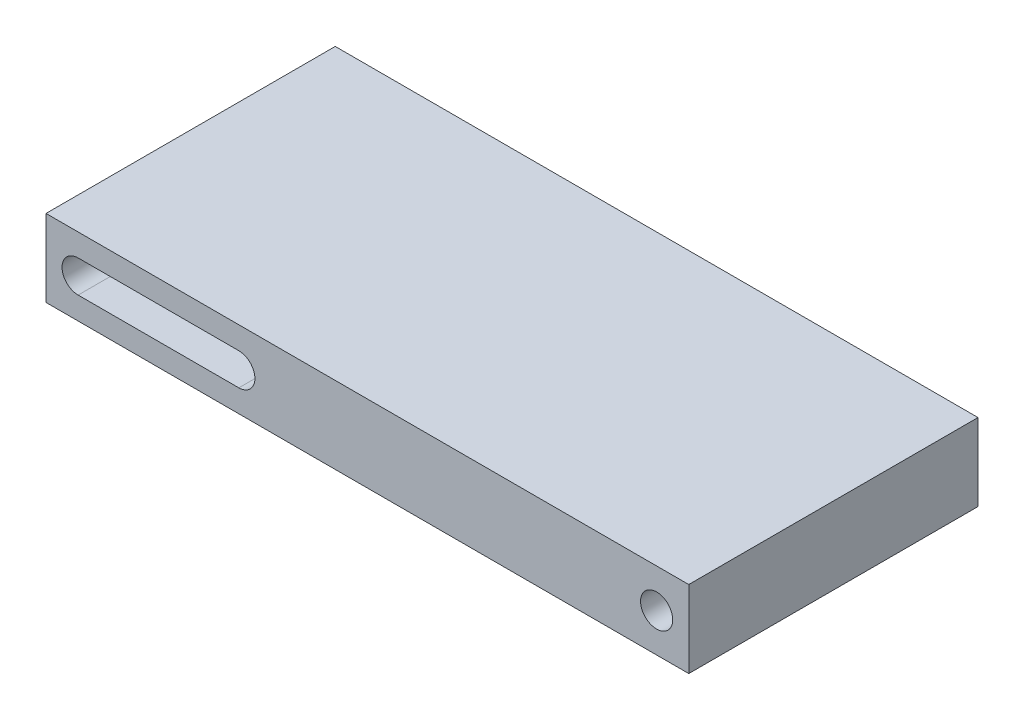
SolidWorks part; units mm, degrees
material "Plain Carbon Steel"
ref_plane "Front Plane" through (0, 0, 0) normal (0, 0, 1) x (1, 0, 0)
ref_plane "Top Plane" through (0, 0, 0) normal (0, 1, 0) x (1, 0, 0)
ref_plane "Right Plane" through (0, 0, 0) normal (1, 0, 0) x (0, 0, -1)
sketch "Plate Profile Sketch" plane through (0, 0, 0) normal (0, 0, 1) x (1, 0, 0)
  line L1 (-50, 6) -> (50, 6)
  line L2 (-50, 6) -> (-50, -6)
  line L3 (-50, -6) -> (50, -6)
  line L4 (50, 6) -> (50, -6)
  line L5 (-50, 6) -> (50, -6) construction
  line L6 (-50, -6) -> (50, 6) construction
  point P0 (0, 0)
  dimension "D1" = 100
  dimension "D2" = 12
extrude "Base Plate 100x12x45" add sketch "Plate Profile Sketch" along normal mid plane 45
sketch "Slot and Hole Sketch" plane through (0, 0, 22.5) normal (0, 0, 1) x (1, 0, 0)
  line L0 (-45, 0) -> (-20, 0) construction
  line L1 (-45, 2.5) -> (-20, 2.5)
  line L2 (-45, -2.5) -> (-20, -2.5)
  line L3 (50, -6) -> (50, 6) construction
  line L4 (-50, -6) -> (50, -6) construction
  arc A0 (-45, 2.5) -> (-45, -2.5) centre (-45, 0) ccw
  arc A1 (-20, -2.5) -> (-20, 2.5) centre (-20, 0) ccw
  circle A2 centre (45, 0) radius 2.5
  point P3 (-32.5, 0)
  dimension "D3" = 2.5
  dimension "D4" = 5
  dimension "D1" = 70
  dimension "D2" = 25
  dimension "D5" = 5
  dimension "D6" = 6
extrude "Through Slot and Hole Cut" cut sketch "Slot and Hole Sketch" against normal up to next
